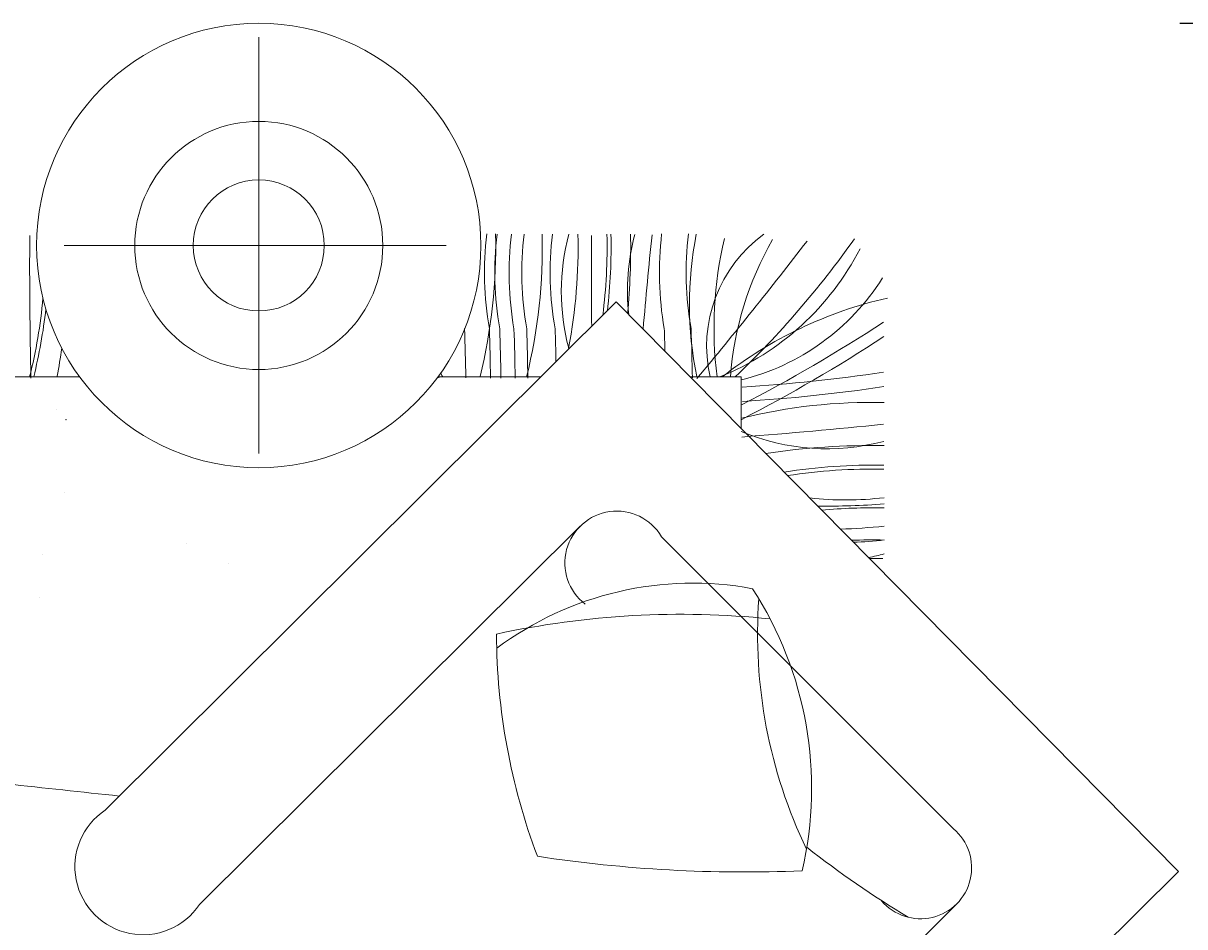
# Model space of a CAD drawing. Units: inches. Extents: x 182 to 1022, y -617 to 111.
# Tile 14 of 33: x 363 to 410, y -250 to -214. Entities that reach past the tile are written whole.
import ezdxf

# ---------------------------------------------------------------- set-up
doc = ezdxf.new("R2010")
doc.units = ezdxf.units.IN
doc.header["$MEASUREMENT"] = 0
doc.layers.add('A-ANNO-DIMS', color=2, linetype='Continuous', lineweight=18)
doc.layers.add('furniture', color=50, linetype='Continuous', lineweight=15, transparency=0.8)
doc.styles.get("Standard").update_dxf_attribs({"font": 'arial.ttf'})
doc.dimstyles.get("Standard").update_dxf_attribs({"dimtxt": 0.18, "dimasz": 0.18, "dimexe": 0.18, "dimexo": 0.0625, "dimgap": 0.09, "dimtad": 0, "dimtih": 1, "dimtoh": 1, "dimdec": 1, "dimzin": 0, "dimdsep": 46, "dimlunit": 4, "dimtxsty": 'Standard', "dimcen": 0.09, "dimadec": 0, "dimazin": 0, "dimtfac": 1, "dimtdec": 1, "dimtofl": 0, "dimtmove": 0, "dimatfit": 3, "dimfxl": 1, "dimtolj": 1, "dimtzin": 0, "dimarcsym": 0})

# ---------------------------------------------------------------- blocks, each defined once
blk = doc.blocks.new('LOUNGE-SEATING-GROUP')
for p, q in [((114.938, 73.887), (114.938, 82.169)), ((114.938, 73.887), (107.197, 73.887)), ((114.938, 73.887), (114.938, 65.605)), ((114.938, 73.887), (122.392, 73.887)), ((129.166, 71.638), (108.826, 51.416)), ((129.166, 71.638), (151.54, 48.98)), ((132.356, 70.43), (132.356, 70.43)), ((132.356, 70.43), (132.356, 70.43)), ((132.356, 70.43), (132.356, 70.43)), ((130.995, 70.096), (130.995, 70.096)), ((130.995, 70.096), (130.995, 70.096)), ((130.995, 70.096), (130.995, 70.096)), ((104.961, 68.655), (107.809, 68.655)), ((122.067, 68.655), (126.166, 68.655)), ((132.112, 68.655), (134.145, 68.655)), ((134.145, 68.655), (134.145, 66.596)), ((106.867, 67.341), (106.867, 67.341)), ((107.192, 64.04), (107.192, 64.04)), ((127.728, 62.711), (112.578, 47.665)), ((112.045, 62.036), (112.045, 62.036)), ((130.966, 62.297), (142.589, 50.675)), ((130.966, 62.297), (132.83, 60.434)), ((106.321, 61.59), (106.321, 61.59)), ((113.723, 61.224), (113.723, 61.224)), ((106.19, 59.881), (106.19, 59.881)), ((136.107, 57.157), (142.589, 50.675)), ((151.54, 48.98), (131.464, 29.017)), ((125.939, 30.989), (142.717, 47.686))]:
    blk.add_line(p, q)
for radius in [8.843, 4.936, 2.608]:
    blk.add_circle((114.938, 73.887), radius)
for centre, radius, start, end in [((290.339, 73.02), 184.521, 179.60659, 181.37204), ((102.817, 73.829), 21.554, 346.1427, 1.3669), ((136.713, 72.811), 12.794, 173.1171, 190.0651), ((137.128, 72.809), 12.794, 173.1171, 190.0651), ((137.693, 72.808), 12.794, 173.1171, 190.0651), ((138.199, 72.807), 12.794, 173.1171, 190.0651), ((104.671, 73.824), 21.554, 346.1427, 1.3669), ((139.33, 72.804), 12.794, 173.1171, 190.0651), ((135.817, 72.065), 8.837, 165.1387, 194.8341), ((106.096, 73.82), 21.554, 349.2534, 1.3669), ((312.696, 73.02), 184.521, 179.60659, 180.73035), ((107.248, 73.818), 21.554, 352.7707, 1.3669), ((107.408, 73.818), 21.554, 353.2584, 1.3669), ((138.45, 72.061), 8.837, 165.1387, 186.0041), ((101.122, 73.849), 28.62, 354.6488, 0.9805), ((380.897, 48.878), 251.596, 174.19829, 175.05746), ((143.676, 72.816), 12.794, 173.1171, 190.0651), ((144.745, 72.813), 12.794, 173.1171, 190.0651), ((146.412, 71.547), 14.333, 168.7545, 191.5888), ((-1.664, 180.448), 174.582, 320.15682, 322.45592), ((138.27, 69.875), 5.505, 125.9057, 192.8054), ((148.602, 70.59), 15.545, 166.7215, 187.1491), ((146.596, 67.692), 12.919, 150.135, 175.7243), ((107.632, 96.133), 38.017, 313.716, 324.6847), ((129.187, 78.752), 10.899, 292.1181, 332.6967), ((131.901, 77.56), 9.302, 283.9935, 327.7288), ((84.891, 73.818), 21.554, 346.1427, 354.5854), ((143.715, 55.463), 16.759, 102.9523, 128.0769), ((85.051, 73.818), 21.554, 346.1427, 353.4467), ((105.088, 123.926), 63.435, 297.26685, 303.17806), ((-19.513, 66.067), 142.714, 1.02248, 1.81091), ((-18.527, 66.065), 142.714, 1.02248, 1.81091), ((-18.112, 66.064), 142.714, 1.02248, 1.81091), ((-17.547, 66.062), 142.714, 1.02248, 1.81091), ((-17.041, 66.061), 142.714, 1.02248, 1.81091), ((-15.91, 66.058), 142.714, 1.2964, 1.81091), ((-11.564, 66.07), 142.714, 1.46162, 1.81091), ((-10.495, 66.067), 142.714, 1.02248, 1.81091), ((105.102, 123.353), 63.435, 297.26685, 303.17806), ((78.765, 73.849), 28.62, 349.5961, 351.862), ((-20.582, 66.07), 142.714, 1.02248, 1.06056), ((130.398, 72.079), 8.837, 201.652, 202.6902), ((130.566, 129.758), 61.61, 273.36442, 278.62286), ((130.58, 129.185), 61.61, 273.36442, 278.62286), ((139.318, 46.088), 21.554, 88.6331, 103.8573), ((114.367, 317.08), 251.596, 274.51462, 275.80171), ((137.55, 74.633), 8.837, 247.3098, 284.8613), ((139.339, 37.305), 28.62, 89.0195, 98.4847), ((139.307, 43.591), 21.554, 88.6331, 99.2236), ((139.308, 43.431), 21.554, 88.6331, 98.8561), ((138.293, 76.552), 12.794, 263.6069, 276.8829), ((137.543, 92.629), 29.116, 269.2987, 274.5064), ((139.313, 41.892), 21.554, 88.6331, 95.2422), ((129.187, 61.25), 2.065, 30.4819, 232.3252), ((137.592, 82.536), 19.942, 271.4332, 276.4413), ((139.323, 40.617), 21.554, 88.6331, 92.1135), ((138.299, 74.87), 12.794, 271.3666, 276.8829), ((137.568, 70.154), 8.837, 280.6792, 284.8613), ((138.51, 245.95), 184.521, 270.22836, 270.39341), ((132.208, 47.417), 13.032, 79.4501, 126.7699), ((122.338, 52.286), 14.605, 347.0126, 32.9429), ((154.559, 58.419), 19.767, 175.9005, 205.6513), ((131.736, 24.698), 34.512, 84.0815, 102.2768), ((149.954, 58.557), 25.556, 180.3068, 200.5663), ((219.704, 1090.605), 1044.469, 263.689239, 263.937357), ((110.325, 49.163), 2.706, 123.6335, 326.3665), ((141.281, 49.122), 2.031, 220.1092, 49.8908), ((161.32, 81.208), 39.767, 231.8457, 238.9133), ((134.263, 103.636), 54.68, 261.3371, 272.4176)]:
    blk.add_arc(centre, radius, start, end)
blk.add_point((107.259, 66.948))
blk = doc.blocks.new('*D27')
at = {"layer": 'A-ANNO-DIMS', "color": 0, "lineweight": -2, "transparency": 16777216}
for p, q in [((409.45, -214.092), (432.299, -214.092)), ((432.119, -214.272), (432.119, -255.274)), ((432.119, -296.642), (432.119, -255.64)), ((409.45, -296.822), (432.299, -296.822))]:
    blk.add_line(p, q, dxfattribs=at)
at = {"layer": 'A-ANNO-DIMS', "color": 0, "transparency": 16777216}
for points in [[(432.089, -214.272), (432.149, -214.272), (432.119, -214.092)], [(432.089, -296.642), (432.149, -296.642), (432.119, -296.822)]]:
    blk.add_solid(points, dxfattribs=at)
at = {"layer": 'Defpoints', "color": 0, "transparency": 16777216}
for p in [(409.388, -214.092), (432.119, -214.092), (409.388, -296.822)]:
    blk.add_point(p, dxfattribs=at)
at = {"layer": 'A-ANNO-DIMS', "color": 0, "transparency": 16777216, "insert": (432.119, -255.457), "char_height": 0.18, "attachment_point": 5}
blk.add_mtext('\\A1;6\'-10 1/2" TYP.', dxfattribs=at)

msp = doc.modelspace()

# ---------------------------------------------------------------- block references
at = {"layer": 'furniture'}
msp.add_blockref('LOUNGE-SEATING-GROUP', (257.848, -296.822), dxfattribs=at)

# ---------------------------------------------------------------- dimensions: what is measured, and where the dimension line sits
at = {"layer": 'A-ANNO-DIMS'}
dim = msp.add_linear_dim(base=(432.119, -214.092), p1=(409.388, -296.822), p2=(409.388, -214.092), angle=90, text='<> TYP.', dimstyle='Standard', override={"dimdec": 1, "dimlfac": 1, "dimrnd": 0, "dimzin": 1, "dimdsep": 46, "dimlunit": 4, "dimfrac": 2}, dxfattribs=at)
dim.commit()
dim.dimension.update_dxf_attribs({"geometry": '*D27', "text_midpoint": (432.119, -255.457)})

doc.saveas('drawing.dxf')
